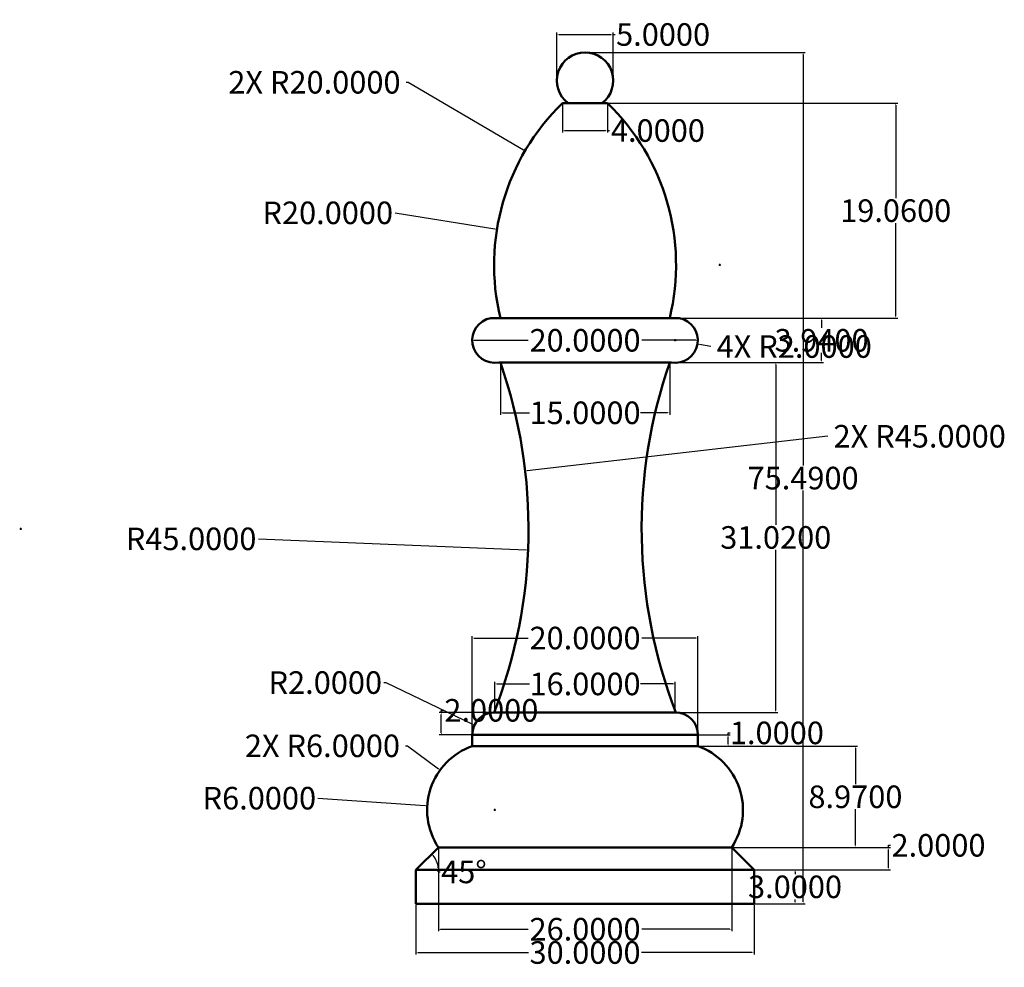
# Model space of a CAD drawing. Units: inches. Extents: x 2555.6 to 2642.8, y 681.4 to 765.4.
import ezdxf

# ---------------------------------------------------------------- set-up
doc = ezdxf.new("R2010")
doc.units = ezdxf.units.IN
doc.header["$MEASUREMENT"] = 0
doc.layers.add('M-DIMS', color=2, linetype='Continuous', lineweight=25)
doc.layers.add('M-OUTL', color=7, linetype='Continuous', lineweight=50)
doc.styles.get("Standard").update_dxf_attribs({"font": 'arial.ttf'})
doc.dimstyles.get("Standard").update_dxf_attribs({"dimtxt": 2, "dimasz": 0.18, "dimexe": 0.18, "dimexo": 0.0625, "dimgap": 0.09, "dimtad": 0, "dimtih": 1, "dimtoh": 1, "dimdec": 4, "dimzin": 0, "dimdsep": 46, "dimtxsty": 'Standard', "dimcen": 0.09, "dimadec": 0, "dimazin": 0, "dimtfac": 1, "dimtdec": 4, "dimtofl": 0, "dimtmove": 0, "dimatfit": 3, "dimfxl": 1, "dimtolj": 1, "dimtzin": 0, "dimarcsym": 0})

# ---------------------------------------------------------------- blocks, each defined once
blk = doc.blocks.new('*D1')
at = {"layer": 'Defpoints', "color": 0, "transparency": 16777216}
for p in [(2555.668, 720.265), (2600.629, 718.391)]:
    blk.add_point(p, dxfattribs=at)
at = {"layer": 'M-DIMS', "color": 0, "lineweight": -2, "transparency": 16777216}
blk.add_line((2576.739, 719.387), (2600.449, 718.399), dxfattribs=at)
at = {"layer": 'M-DIMS', "color": 0, "transparency": 16777216}
blk.add_solid([(2600.451, 718.429), (2600.448, 718.369), (2600.629, 718.391)], dxfattribs=at)
at = {"layer": 'M-DIMS', "color": 0, "transparency": 16777216, "insert": (2570.767, 719.387), "char_height": 2, "attachment_point": 5}
blk.add_mtext('\\A1;R45.0000', dxfattribs=at)
blk = doc.blocks.new('*D2')
at = {"layer": 'Defpoints', "color": 0, "transparency": 16777216}
for p in [(2597.869, 746.846), (2617.616, 743.676)]:
    blk.add_point(p, dxfattribs=at)
at = {"layer": 'M-DIMS', "color": 0, "lineweight": -2, "transparency": 16777216}
for p, q in [((2588.849, 748.294), (2597.691, 746.875)), ((2617.526, 743.676), (2617.706, 743.676)), ((2617.616, 743.586), (2617.616, 743.766))]:
    blk.add_line(p, q, dxfattribs=at)
at = {"layer": 'M-DIMS', "color": 0, "transparency": 16777216}
blk.add_solid([(2597.696, 746.904), (2597.687, 746.845), (2597.869, 746.846)], dxfattribs=at)
at = {"layer": 'M-DIMS', "color": 0, "transparency": 16777216, "insert": (2582.877, 748.294), "char_height": 2, "attachment_point": 5}
blk.add_mtext('\\A1;R20.0000', dxfattribs=at)
blk = doc.blocks.new('*D3')
at = {"layer": 'Defpoints', "color": 0, "transparency": 16777216}
for p in [(2595.878, 702.869), (2597.68, 702.001)]:
    blk.add_point(p, dxfattribs=at)
at = {"layer": 'M-DIMS', "color": 0, "lineweight": -2, "transparency": 16777216}
for p, q in [((2587.855, 706.643), (2588.035, 706.643)), ((2588.035, 706.643), (2595.716, 702.947)), ((2597.59, 702.001), (2597.77, 702.001)), ((2597.68, 701.911), (2597.68, 702.091))]:
    blk.add_line(p, q, dxfattribs=at)
at = {"layer": 'M-DIMS', "color": 0, "transparency": 16777216}
blk.add_solid([(2595.729, 702.974), (2595.703, 702.92), (2595.878, 702.869)], dxfattribs=at)
at = {"layer": 'M-DIMS', "color": 0, "transparency": 16777216, "insert": (2582.66, 706.643), "char_height": 2, "attachment_point": 5}
blk.add_mtext('\\A1;R2.0000', dxfattribs=at)
blk = doc.blocks.new('*D4')
at = {"layer": 'Defpoints', "color": 0, "transparency": 16777216}
for p in [(2591.695, 695.745), (2597.682, 695.345)]:
    blk.add_point(p, dxfattribs=at)
at = {"layer": 'M-DIMS', "color": 0, "lineweight": -2, "transparency": 16777216}
for p, q in [((2582.01, 696.392), (2591.516, 695.757)), ((2597.682, 695.255), (2597.682, 695.435)), ((2597.592, 695.345), (2597.772, 695.345))]:
    blk.add_line(p, q, dxfattribs=at)
at = {"layer": 'M-DIMS', "color": 0, "transparency": 16777216}
blk.add_solid([(2591.518, 695.787), (2591.514, 695.727), (2591.695, 695.745)], dxfattribs=at)
at = {"layer": 'M-DIMS', "color": 0, "transparency": 16777216, "insert": (2576.815, 696.392), "char_height": 2, "attachment_point": 5}
blk.add_mtext('\\A1;R6.0000', dxfattribs=at)
blk = doc.blocks.new('*D5')
at = {"layer": 'Defpoints', "color": 0, "transparency": 16777216}
for p in [(2592.68, 692.031), (2618.68, 692.031), (2618.68, 684.769)]:
    blk.add_point(p, dxfattribs=at)
at = {"layer": 'M-DIMS', "color": 0, "lineweight": -2, "transparency": 16777216}
for p, q in [((2592.68, 691.969), (2592.68, 684.589)), ((2618.68, 691.969), (2618.68, 684.589)), ((2592.86, 684.769), (2600.648, 684.769)), ((2618.5, 684.769), (2610.712, 684.769))]:
    blk.add_line(p, q, dxfattribs=at)
at = {"layer": 'M-DIMS', "color": 0, "transparency": 16777216}
for points in [[(2592.86, 684.799), (2592.86, 684.739), (2592.68, 684.769)], [(2618.5, 684.799), (2618.5, 684.739), (2618.68, 684.769)]]:
    blk.add_solid(points, dxfattribs=at)
at = {"layer": 'M-DIMS', "color": 0, "transparency": 16777216, "insert": (2605.68, 684.769), "char_height": 2, "attachment_point": 5}
blk.add_mtext('\\A1;26.0000', dxfattribs=at)
blk = doc.blocks.new('*D6')
at = {"layer": 'Defpoints', "color": 0, "transparency": 16777216}
for p in [(2605.68, 735.021), (2622.58, 735.021), (2605.68, 704.001)]:
    blk.add_point(p, dxfattribs=at)
at = {"layer": 'M-DIMS', "color": 0, "lineweight": -2, "transparency": 16777216}
for p, q in [((2605.743, 735.021), (2622.76, 735.021)), ((2622.58, 734.841), (2622.58, 720.623)), ((2622.58, 704.181), (2622.58, 718.399)), ((2605.743, 704.001), (2622.76, 704.001))]:
    blk.add_line(p, q, dxfattribs=at)
at = {"layer": 'M-DIMS', "color": 0, "transparency": 16777216}
for points in [[(2622.55, 734.841), (2622.61, 734.841), (2622.58, 735.021)], [(2622.55, 704.181), (2622.61, 704.181), (2622.58, 704.001)]]:
    blk.add_solid(points, dxfattribs=at)
at = {"layer": 'M-DIMS', "color": 0, "transparency": 16777216, "insert": (2622.58, 719.511), "char_height": 2, "attachment_point": 5}
blk.add_mtext('\\A1;31.0200', dxfattribs=at)
blk = doc.blocks.new('*D7')
at = {"layer": 'Defpoints', "color": 0, "transparency": 16777216}
for p in [(2605.68, 701.001), (2629.641, 701.001), (2605.68, 692.031)]:
    blk.add_point(p, dxfattribs=at)
at = {"layer": 'M-DIMS', "color": 0, "lineweight": -2, "transparency": 16777216}
for p, q in [((2605.743, 701.001), (2629.821, 701.001)), ((2629.641, 700.821), (2629.641, 697.627)), ((2629.641, 692.211), (2629.641, 695.405)), ((2605.743, 692.031), (2629.821, 692.031))]:
    blk.add_line(p, q, dxfattribs=at)
at = {"layer": 'M-DIMS', "color": 0, "transparency": 16777216}
for points in [[(2629.611, 700.821), (2629.671, 700.821), (2629.641, 701.001)], [(2629.611, 692.211), (2629.671, 692.211), (2629.641, 692.031)]]:
    blk.add_solid(points, dxfattribs=at)
at = {"layer": 'M-DIMS', "color": 0, "transparency": 16777216, "insert": (2629.641, 696.516), "char_height": 2, "attachment_point": 5}
blk.add_mtext('\\A1;8.9700', dxfattribs=at)
blk = doc.blocks.new('*D8')
at = {"layer": 'Defpoints', "color": 0, "transparency": 16777216}
for p in [(2615.767, 692.031), (2632.569, 692.031), (2615.767, 690.031)]:
    blk.add_point(p, dxfattribs=at)
at = {"layer": 'M-DIMS', "color": 0, "lineweight": -2, "transparency": 16777216}
for p, q in [((2615.829, 692.031), (2632.749, 692.031)), ((2632.569, 692.031), (2632.569, 692.211)), ((2632.569, 692.211), (2632.749, 692.211)), ((2632.569, 690.211), (2632.569, 691.851)), ((2615.829, 690.031), (2632.749, 690.031))]:
    blk.add_line(p, q, dxfattribs=at)
at = {"layer": 'M-DIMS', "color": 0, "transparency": 16777216}
for points in [[(2632.539, 691.851), (2632.599, 691.851), (2632.569, 692.031)], [(2632.539, 690.211), (2632.599, 690.211), (2632.569, 690.031)]]:
    blk.add_solid(points, dxfattribs=at)
at = {"layer": 'M-DIMS', "color": 0, "transparency": 16777216, "insert": (2637.004, 692.211), "char_height": 2, "attachment_point": 5}
blk.add_mtext('\\A1;2.0000', dxfattribs=at)
blk = doc.blocks.new('*D9')
at = {"layer": 'Defpoints', "color": 0, "transparency": 16777216}
for p in [(2620.68, 690.031), (2624.289, 690.031), (2620.68, 687.031)]:
    blk.add_point(p, dxfattribs=at)
at = {"layer": 'M-DIMS', "color": 0, "lineweight": -2, "transparency": 16777216}
for p, q in [((2620.743, 690.031), (2624.469, 690.031)), ((2624.289, 689.851), (2624.289, 689.643)), ((2620.743, 687.031), (2624.469, 687.031)), ((2624.289, 687.211), (2624.289, 687.419))]:
    blk.add_line(p, q, dxfattribs=at)
at = {"layer": 'M-DIMS', "color": 0, "transparency": 16777216}
for points in [[(2624.259, 689.851), (2624.319, 689.851), (2624.289, 690.031)], [(2624.259, 687.211), (2624.319, 687.211), (2624.289, 687.031)]]:
    blk.add_solid(points, dxfattribs=at)
at = {"layer": 'M-DIMS', "color": 0, "transparency": 16777216, "insert": (2624.289, 688.531), "char_height": 2, "attachment_point": 5}
blk.add_mtext('\\A1;3.0000', dxfattribs=at)
blk = doc.blocks.new('*D10')
at = {"layer": 'Defpoints', "color": 0, "transparency": 16777216}
for p in [(2605.68, 738.961), (2626.643, 738.961), (2605.68, 735.021)]:
    blk.add_point(p, dxfattribs=at)
at = {"layer": 'M-DIMS', "color": 0, "lineweight": -2, "transparency": 16777216}
for p, q in [((2605.743, 738.961), (2626.823, 738.961)), ((2626.643, 738.781), (2626.643, 738.103)), ((2626.643, 735.201), (2626.643, 735.879)), ((2605.743, 735.021), (2626.823, 735.021))]:
    blk.add_line(p, q, dxfattribs=at)
at = {"layer": 'M-DIMS', "color": 0, "transparency": 16777216}
for points in [[(2626.613, 738.781), (2626.673, 738.781), (2626.643, 738.961)], [(2626.613, 735.201), (2626.673, 735.201), (2626.643, 735.021)]]:
    blk.add_solid(points, dxfattribs=at)
at = {"layer": 'M-DIMS', "color": 0, "transparency": 16777216, "insert": (2626.643, 736.991), "char_height": 2, "attachment_point": 5}
blk.add_mtext('\\A1;3.9400', dxfattribs=at)
blk = doc.blocks.new('*D11')
at = {"layer": 'Defpoints', "color": 0, "transparency": 16777216}
for p in [(2605.68, 758.021), (2633.212, 758.021), (2605.68, 738.961)]:
    blk.add_point(p, dxfattribs=at)
at = {"layer": 'M-DIMS', "color": 0, "lineweight": -2, "transparency": 16777216}
for p, q in [((2605.743, 758.021), (2633.392, 758.021)), ((2633.212, 757.841), (2633.212, 749.602)), ((2633.212, 739.141), (2633.212, 747.38)), ((2605.743, 738.961), (2633.392, 738.961))]:
    blk.add_line(p, q, dxfattribs=at)
at = {"layer": 'M-DIMS', "color": 0, "transparency": 16777216}
for points in [[(2633.182, 757.841), (2633.242, 757.841), (2633.212, 758.021)], [(2633.182, 739.141), (2633.242, 739.141), (2633.212, 738.961)]]:
    blk.add_solid(points, dxfattribs=at)
at = {"layer": 'M-DIMS', "color": 0, "transparency": 16777216, "insert": (2633.212, 748.491), "char_height": 2, "attachment_point": 5}
blk.add_mtext('\\A1;19.0600', dxfattribs=at)
blk = doc.blocks.new('*D12')
at = {"layer": 'Defpoints', "color": 0, "transparency": 16777216}
for p in [(2608.18, 764.109), (2603.18, 760.021), (2608.18, 760.021)]:
    blk.add_point(p, dxfattribs=at)
at = {"layer": 'M-DIMS', "color": 0, "lineweight": -2, "transparency": 16777216}
for p, q in [((2603.18, 760.084), (2603.18, 764.289)), ((2603.36, 764.109), (2608, 764.109)), ((2608.18, 760.084), (2608.18, 764.289)), ((2608.18, 764.109), (2608.36, 764.109))]:
    blk.add_line(p, q, dxfattribs=at)
at = {"layer": 'M-DIMS', "color": 0, "transparency": 16777216}
for points in [[(2603.36, 764.139), (2603.36, 764.079), (2603.18, 764.109)], [(2608, 764.139), (2608, 764.079), (2608.18, 764.109)]]:
    blk.add_solid(points, dxfattribs=at)
at = {"layer": 'M-DIMS', "color": 0, "transparency": 16777216, "insert": (2612.598, 764.109), "char_height": 2, "attachment_point": 5}
blk.add_mtext('\\A1;5.0000', dxfattribs=at)
blk = doc.blocks.new('*D13')
at = {"layer": 'Defpoints', "color": 0, "transparency": 16777216}
for p in [(2598.18, 735.021), (2613.18, 735.021), (2613.18, 730.565)]:
    blk.add_point(p, dxfattribs=at)
at = {"layer": 'M-DIMS', "color": 0, "lineweight": -2, "transparency": 16777216}
for p, q in [((2598.18, 734.959), (2598.18, 730.385)), ((2613.18, 734.959), (2613.18, 730.385)), ((2598.36, 730.565), (2600.759, 730.565)), ((2613, 730.565), (2610.601, 730.565))]:
    blk.add_line(p, q, dxfattribs=at)
at = {"layer": 'M-DIMS', "color": 0, "transparency": 16777216}
for points in [[(2598.36, 730.595), (2598.36, 730.535), (2598.18, 730.565)], [(2613, 730.595), (2613, 730.535), (2613.18, 730.565)]]:
    blk.add_solid(points, dxfattribs=at)
at = {"layer": 'M-DIMS', "color": 0, "transparency": 16777216, "insert": (2605.68, 730.565), "char_height": 2, "attachment_point": 5}
blk.add_mtext('\\A1;15.0000', dxfattribs=at)
blk = doc.blocks.new('*D14')
at = {"layer": 'Defpoints', "color": 0, "transparency": 16777216}
for p in [(2595.68, 736.991), (2615.68, 736.991), (2615.68, 736.991)]:
    blk.add_point(p, dxfattribs=at)
at = {"layer": 'M-DIMS', "color": 0, "lineweight": -2, "transparency": 16777216}
for p, q in [((2595.68, 737.054), (2595.68, 737.171)), ((2595.86, 736.991), (2600.648, 736.991)), ((2615.5, 736.991), (2610.712, 736.991)), ((2615.68, 737.054), (2615.68, 737.171))]:
    blk.add_line(p, q, dxfattribs=at)
at = {"layer": 'M-DIMS', "color": 0, "transparency": 16777216}
for points in [[(2595.86, 737.021), (2595.86, 736.961), (2595.68, 736.991)], [(2615.5, 737.021), (2615.5, 736.961), (2615.68, 736.991)]]:
    blk.add_solid(points, dxfattribs=at)
at = {"layer": 'M-DIMS', "color": 0, "transparency": 16777216, "insert": (2605.68, 736.991), "char_height": 2, "attachment_point": 5}
blk.add_mtext('\\A1;20.0000', dxfattribs=at)
blk = doc.blocks.new('*D15')
at = {"layer": 'Defpoints', "color": 0, "transparency": 16777216}
for p in [(2613.68, 706.522), (2597.68, 704.001), (2613.68, 704.001)]:
    blk.add_point(p, dxfattribs=at)
at = {"layer": 'M-DIMS', "color": 0, "lineweight": -2, "transparency": 16777216}
for p, q in [((2597.68, 704.064), (2597.68, 706.702)), ((2597.86, 706.522), (2600.759, 706.522)), ((2613.5, 706.522), (2610.601, 706.522)), ((2613.68, 704.064), (2613.68, 706.702))]:
    blk.add_line(p, q, dxfattribs=at)
at = {"layer": 'M-DIMS', "color": 0, "transparency": 16777216}
for points in [[(2597.86, 706.552), (2597.86, 706.492), (2597.68, 706.522)], [(2613.5, 706.552), (2613.5, 706.492), (2613.68, 706.522)]]:
    blk.add_solid(points, dxfattribs=at)
at = {"layer": 'M-DIMS', "color": 0, "transparency": 16777216, "insert": (2605.68, 706.522), "char_height": 2, "attachment_point": 5}
blk.add_mtext('\\A1;16.0000', dxfattribs=at)
blk = doc.blocks.new('*D16')
at = {"layer": 'Defpoints', "color": 0, "transparency": 16777216}
for p in [(2615.68, 710.592), (2595.68, 702.001), (2615.68, 702.001)]:
    blk.add_point(p, dxfattribs=at)
at = {"layer": 'M-DIMS', "color": 0, "lineweight": -2, "transparency": 16777216}
for p, q in [((2595.68, 702.064), (2595.68, 710.772)), ((2595.86, 710.592), (2600.648, 710.592)), ((2615.5, 710.592), (2610.712, 710.592)), ((2615.68, 702.064), (2615.68, 710.772))]:
    blk.add_line(p, q, dxfattribs=at)
at = {"layer": 'M-DIMS', "color": 0, "transparency": 16777216}
for points in [[(2595.86, 710.622), (2595.86, 710.562), (2595.68, 710.592)], [(2615.5, 710.622), (2615.5, 710.562), (2615.68, 710.592)]]:
    blk.add_solid(points, dxfattribs=at)
at = {"layer": 'M-DIMS', "color": 0, "transparency": 16777216, "insert": (2605.68, 710.592), "char_height": 2, "attachment_point": 5}
blk.add_mtext('\\A1;20.0000', dxfattribs=at)
blk = doc.blocks.new('*D17')
at = {"layer": 'Defpoints', "color": 0, "transparency": 16777216}
for p in [(2592.68, 692.031), (2592.412, 691.031), (2590.68, 690.031), (2590.68, 690.031), (2620.68, 690.031)]:
    blk.add_point(p, dxfattribs=at)
at = {"layer": 'M-DIMS', "color": 0, "lineweight": -2, "transparency": 16777216}
blk.add_line((2592.672, 689.852), (2592.852, 689.852), dxfattribs=at)
for start, end in [(5.15836, 39.84164), (354.84164, 360)]:
    blk.add_arc((2590.68, 690.031), 2, start, end, dxfattribs=at)
at = {"layer": 'M-DIMS', "color": 0, "transparency": 16777216}
for points in [[(2592.194, 691.292), (2592.238, 691.333), (2592.094, 691.446)], [(2592.702, 690.212), (2592.642, 690.21), (2592.68, 690.031)]]:
    blk.add_solid(points, dxfattribs=at)
at = {"layer": 'M-DIMS', "color": 0, "transparency": 16777216, "insert": (2594.944, 689.852), "char_height": 2, "attachment_point": 5}
blk.add_mtext('\\A1;45°', dxfattribs=at)
blk = doc.blocks.new('*D18')
at = {"layer": 'Defpoints', "color": 0, "transparency": 16777216}
for p in [(2615.68, 702.001), (2618.355, 702.001), (2615.68, 701.001)]:
    blk.add_point(p, dxfattribs=at)
at = {"layer": 'M-DIMS', "color": 0, "lineweight": -2, "transparency": 16777216}
for p, q in [((2615.743, 702.001), (2618.535, 702.001)), ((2618.355, 702.001), (2618.355, 702.181)), ((2618.355, 702.181), (2618.535, 702.181)), ((2618.355, 701.181), (2618.355, 701.821)), ((2615.743, 701.001), (2618.535, 701.001))]:
    blk.add_line(p, q, dxfattribs=at)
at = {"layer": 'M-DIMS', "color": 0, "transparency": 16777216}
for points in [[(2618.325, 701.821), (2618.385, 701.821), (2618.355, 702.001)], [(2618.325, 701.181), (2618.385, 701.181), (2618.355, 701.001)]]:
    blk.add_solid(points, dxfattribs=at)
at = {"layer": 'M-DIMS', "color": 0, "transparency": 16777216, "insert": (2622.679, 702.181), "char_height": 2, "attachment_point": 5}
blk.add_mtext('\\A1;1.0000', dxfattribs=at)
blk = doc.blocks.new('*D19')
at = {"layer": 'Defpoints', "color": 0, "transparency": 16777216}
for p in [(2592.943, 704.001), (2604.037, 704.001), (2604.037, 702.001)]:
    blk.add_point(p, dxfattribs=at)
at = {"layer": 'M-DIMS', "color": 0, "lineweight": -2, "transparency": 16777216}
for p, q in [((2592.943, 704.001), (2592.943, 704.181)), ((2592.943, 704.181), (2593.123, 704.181)), ((2603.975, 704.001), (2592.763, 704.001)), ((2592.943, 702.181), (2592.943, 703.821)), ((2603.975, 702.001), (2592.763, 702.001))]:
    blk.add_line(p, q, dxfattribs=at)
at = {"layer": 'M-DIMS', "color": 0, "transparency": 16777216}
for points in [[(2592.913, 703.821), (2592.973, 703.821), (2592.943, 704.001)], [(2592.913, 702.181), (2592.973, 702.181), (2592.943, 702.001)]]:
    blk.add_solid(points, dxfattribs=at)
at = {"layer": 'M-DIMS', "color": 0, "transparency": 16777216, "insert": (2597.378, 704.181), "char_height": 2, "attachment_point": 5}
blk.add_mtext('\\A1;2.0000', dxfattribs=at)
blk = doc.blocks.new('*D20')
at = {"layer": 'Defpoints', "color": 0, "transparency": 16777216}
for p in [(2603.68, 758.021), (2607.68, 758.021), (2607.68, 755.591)]:
    blk.add_point(p, dxfattribs=at)
at = {"layer": 'M-DIMS', "color": 0, "lineweight": -2, "transparency": 16777216}
for p, q in [((2603.68, 757.959), (2603.68, 755.411)), ((2607.68, 757.959), (2607.68, 755.411)), ((2603.86, 755.591), (2607.5, 755.591)), ((2607.68, 755.591), (2607.86, 755.591))]:
    blk.add_line(p, q, dxfattribs=at)
at = {"layer": 'M-DIMS', "color": 0, "transparency": 16777216}
for points in [[(2603.86, 755.621), (2603.86, 755.561), (2603.68, 755.591)], [(2607.5, 755.621), (2607.5, 755.561), (2607.68, 755.591)]]:
    blk.add_solid(points, dxfattribs=at)
at = {"layer": 'M-DIMS', "color": 0, "transparency": 16777216, "insert": (2612.138, 755.591), "char_height": 2, "attachment_point": 5}
blk.add_mtext('\\A1;4.0000', dxfattribs=at)
blk = doc.blocks.new('*D21')
at = {"layer": 'Defpoints', "color": 0, "transparency": 16777216}
for p in [(2605.68, 762.521), (2620.68, 687.031), (2625.005, 687.031)]:
    blk.add_point(p, dxfattribs=at)
at = {"layer": 'M-DIMS', "color": 0, "lineweight": -2, "transparency": 16777216}
for p, q in [((2605.743, 762.521), (2625.185, 762.521)), ((2625.005, 762.341), (2625.005, 725.887)), ((2625.005, 687.211), (2625.005, 723.665)), ((2620.743, 687.031), (2625.185, 687.031))]:
    blk.add_line(p, q, dxfattribs=at)
at = {"layer": 'M-DIMS', "color": 0, "transparency": 16777216}
for points in [[(2624.975, 762.341), (2625.035, 762.341), (2625.005, 762.521)], [(2624.975, 687.211), (2625.035, 687.211), (2625.005, 687.031)]]:
    blk.add_solid(points, dxfattribs=at)
at = {"layer": 'M-DIMS', "color": 0, "transparency": 16777216, "insert": (2625.005, 724.776), "char_height": 2, "attachment_point": 5}
blk.add_mtext('\\A1;75.4900', dxfattribs=at)
blk = doc.blocks.new('*D22')
at = {"layer": 'Defpoints', "color": 0, "transparency": 16777216}
for p in [(2590.68, 687.031), (2620.68, 687.031), (2620.68, 682.706)]:
    blk.add_point(p, dxfattribs=at)
at = {"layer": 'M-DIMS', "color": 0, "lineweight": -2, "transparency": 16777216}
for p, q in [((2590.68, 686.969), (2590.68, 682.526)), ((2620.68, 686.969), (2620.68, 682.526)), ((2590.86, 682.706), (2600.666, 682.706)), ((2620.5, 682.706), (2610.694, 682.706))]:
    blk.add_line(p, q, dxfattribs=at)
at = {"layer": 'M-DIMS', "color": 0, "transparency": 16777216}
for points in [[(2590.86, 682.736), (2590.86, 682.676), (2590.68, 682.706)], [(2620.5, 682.736), (2620.5, 682.676), (2620.68, 682.706)]]:
    blk.add_solid(points, dxfattribs=at)
at = {"layer": 'M-DIMS', "color": 0, "transparency": 16777216, "insert": (2605.68, 682.706), "char_height": 2, "attachment_point": 5}
blk.add_mtext('\\A1;30.0000', dxfattribs=at)
blk = doc.blocks.new('*D23')
at = {"layer": 'Defpoints', "color": 0, "transparency": 16777216}
for p in [(2600.366, 753.797), (2617.616, 743.676)]:
    blk.add_point(p, dxfattribs=at)
at = {"layer": 'M-DIMS', "color": 0, "lineweight": -2, "transparency": 16777216}
for p, q in [((2589.836, 759.87), (2590.016, 759.87)), ((2590.016, 759.87), (2600.211, 753.888)), ((2617.526, 743.676), (2617.706, 743.676)), ((2617.616, 743.586), (2617.616, 743.766))]:
    blk.add_line(p, q, dxfattribs=at)
at = {"layer": 'M-DIMS', "color": 0, "transparency": 16777216}
blk.add_solid([(2600.226, 753.914), (2600.196, 753.862), (2600.366, 753.797)], dxfattribs=at)
at = {"layer": 'M-DIMS', "color": 0, "transparency": 16777216, "insert": (2581.698, 759.87), "char_height": 2, "attachment_point": 5}
blk.add_mtext('\\A1;2X R20.0000', dxfattribs=at)
blk = doc.blocks.new('*D24')
at = {"layer": 'Defpoints', "color": 0, "transparency": 16777216}
for p in [(2600.374, 725.403), (2555.668, 720.265)]:
    blk.add_point(p, dxfattribs=at)
at = {"layer": 'M-DIMS', "color": 0, "lineweight": -2, "transparency": 16777216}
for p, q in [((2627.197, 728.485), (2600.553, 725.423)), ((2555.578, 720.265), (2555.758, 720.265)), ((2555.668, 720.175), (2555.668, 720.355))]:
    blk.add_line(p, q, dxfattribs=at)
at = {"layer": 'M-DIMS', "color": 0, "transparency": 16777216}
blk.add_solid([(2600.549, 725.453), (2600.556, 725.393), (2600.374, 725.403)], dxfattribs=at)
at = {"layer": 'M-DIMS', "color": 0, "transparency": 16777216, "insert": (2635.335, 728.485), "char_height": 2, "attachment_point": 5}
blk.add_mtext('\\A1;2X R45.0000', dxfattribs=at)
blk = doc.blocks.new('*D25')
at = {"layer": 'Defpoints', "color": 0, "transparency": 16777216}
for p in [(2592.849, 698.901), (2597.682, 695.345)]:
    blk.add_point(p, dxfattribs=at)
at = {"layer": 'M-DIMS', "color": 0, "lineweight": -2, "transparency": 16777216}
for p, q in [((2589.769, 701.034), (2589.949, 701.034)), ((2589.949, 701.034), (2592.704, 699.007)), ((2597.682, 695.255), (2597.682, 695.435)), ((2597.592, 695.345), (2597.772, 695.345))]:
    blk.add_line(p, q, dxfattribs=at)
at = {"layer": 'M-DIMS', "color": 0, "transparency": 16777216}
blk.add_solid([(2592.722, 699.032), (2592.686, 698.983), (2592.849, 698.901)], dxfattribs=at)
at = {"layer": 'M-DIMS', "color": 0, "transparency": 16777216, "insert": (2582.408, 701.034), "char_height": 2, "attachment_point": 5}
blk.add_mtext('\\A1;2X R6.0000', dxfattribs=at)
blk = doc.blocks.new('*D26')
at = {"layer": 'Defpoints', "color": 0, "transparency": 16777216}
for p in [(2613.68, 736.991), (2615.65, 736.646)]:
    blk.add_point(p, dxfattribs=at)
at = {"layer": 'M-DIMS', "color": 0, "lineweight": -2, "transparency": 16777216}
for p, q in [((2613.59, 736.991), (2613.77, 736.991)), ((2613.68, 736.901), (2613.68, 737.081)), ((2616.832, 736.439), (2615.827, 736.615))]:
    blk.add_line(p, q, dxfattribs=at)
at = {"layer": 'M-DIMS', "color": 0, "transparency": 16777216}
blk.add_solid([(2615.832, 736.644), (2615.822, 736.585), (2615.65, 736.646)], dxfattribs=at)
at = {"layer": 'M-DIMS', "color": 0, "transparency": 16777216, "insert": (2624.216, 736.439), "char_height": 2, "attachment_point": 5}
blk.add_mtext('\\A1;4X R2.0000', dxfattribs=at)

msp = doc.modelspace()

# ---------------------------------------------------------------- linework, layer by layer
at = {"layer": 'M-OUTL'}
for p, q in [((2603.68005, 758.02133), (2607.68005, 758.02133)), ((2603.68005, 758.02133), (2607.68005, 758.02133)), ((2598.18005, 738.96133), (2597.33495, 738.96133)), ((2598.18005, 738.96133), (2613.18005, 738.96133)), ((2613.18005, 738.96133), (2614.02516, 738.96133)), ((2598.02516, 735.02133), (2613.33495, 735.02133)), ((2597.68005, 704.00133), (2613.68005, 704.00133)), ((2595.68005, 702.00133), (2615.68005, 702.00133)), ((2595.68005, 702.00133), (2595.68005, 701.00133)), ((2615.68005, 702.00133), (2615.68005, 701.00133)), ((2595.68005, 701.00133), (2615.68005, 701.00133)), ((2592.68005, 692.03133), (2590.68005, 690.03133)), ((2592.68005, 692.03133), (2618.68005, 692.03133)), ((2618.68005, 692.03133), (2620.68005, 690.03133)), ((2590.68005, 690.03133), (2620.68005, 690.03133)), ((2590.68005, 690.03133), (2590.68005, 687.03133)), ((2620.68005, 690.03133), (2620.68005, 687.03133)), ((2590.68005, 687.03133), (2592.68005, 687.03133)), ((2592.68005, 687.03133), (2620.68005, 687.03133))]:
    msp.add_line(p, q, dxfattribs=at)
for centre, radius, start, end in [((2605.68005, 760.02133), 2.5, 306.8698976, 233.1301024), ((2617.61634, 743.67629), 20, 134.1719587, 193.6357352), ((2593.74377, 743.67629), 20, 346.3642648, 45.8280413), ((2597.68005, 736.99133), 2, 99.9363671, 279.9363671), ((2613.68005, 736.99133), 2, 260.0636329, 80.0636329), ((2555.66815, 720.26538), 45, 338.8113585, 19.1419619), ((2655.69196, 720.26538), 45, 160.8580381, 201.1886415), ((2597.68005, 702.00133), 2, 90, 180), ((2613.68005, 702.00133), 2, 0, 90), ((2597.68192, 695.34513), 6, 109.4901441, 213.5250219), ((2613.67819, 695.34513), 6, 326.4749781, 70.5098559)]:
    msp.add_arc(centre, radius, start, end, dxfattribs=at)

# ---------------------------------------------------------------- dimensions: what is measured, and where the dimension line sits
at = {"layer": 'M-DIMS'}
for base, p1, p2, override, picture, middle in [((2608.18005, 764.10928), (2603.18005, 760.02133), (2608.18005, 760.02133), {"dimclrd": 0, "dimclre": 0, "dimclrt": 0}, '*D12', (2612.59808, 764.10928)), ((2607.68005, 755.5907), (2603.68005, 758.02133), (2607.68005, 758.02133), {"dimclrd": 0, "dimclre": 0, "dimclrt": 0}, '*D20', (2612.13832, 755.5907)), ((2615.68005, 736.99133), (2595.68005, 736.99133), (2615.68005, 736.99133), {"dimclrd": 0, "dimclre": 0, "dimclrt": 0}, '*D14', (2605.68005, 736.99133)), ((2613.18005, 730.56464), (2598.18005, 735.02133), (2613.18005, 735.02133), {"dimclrd": 0, "dimclre": 0, "dimclrt": 0}, '*D13', (2605.68005, 730.56464)), ((2615.68005, 710.5918), (2595.68005, 702.00133), (2615.68005, 702.00133), {"dimclrd": 0, "dimclre": 0, "dimclrt": 0}, '*D16', (2605.68005, 710.5918)), ((2613.68005, 706.52229), (2597.68005, 704.00133), (2613.68005, 704.00133), {"dimclrd": 0, "dimclre": 0, "dimclrt": 0}, '*D15', (2605.68005, 706.52229)), ((2618.68005, 684.76855), (2592.68005, 692.03133), (2618.68005, 692.03133), {"dimclrd": 0, "dimclre": 0, "dimclrt": 0}, '*D5', (2605.68005, 684.76855)), ((2620.68005, 682.70633), (2590.68005, 687.03133), (2620.68005, 687.03133), {"dimdec": 4, "dimlfac": 1, "dimrnd": 0, "dimzin": 0, "dimdsep": 46, "dimlunit": 2}, '*D22', (2605.68005, 682.70633))]:
    dim = msp.add_linear_dim(base=base, p1=p1, p2=p2, dimstyle='Standard', override=override, dxfattribs=at)
    dim.commit()
    dim.dimension.update_dxf_attribs({"geometry": picture, "text_midpoint": middle})
for center, mpoint, text, picture, middle in [((2617.61634, 743.67629), (2600.36617, 753.79715), '2X <>', '*D23', (2581.69833, 759.86967)), ((2613.68005, 736.99133), (2615.65002, 736.646), '4X <>', '*D26', (2616.83199, 736.4388)), ((2555.66815, 720.26538), (2600.37394, 725.40275), '2X <>', '*D24', (2627.19741, 728.48517)), ((2597.68192, 695.34513), (2592.84896, 698.90076), '2X <>', '*D25', (2582.40838, 701.03414))]:
    dim = msp.add_radius_dim(center=center, mpoint=mpoint, text=text, dimstyle='Standard', override={"dimdec": 4, "dimlfac": 1, "dimrnd": 0, "dimzin": 0, "dimdsep": 46, "dimlunit": 2}, dxfattribs=at)
    dim.commit()
    dim.dimension.update_dxf_attribs({"geometry": picture, "text_midpoint": middle, "dimtype": 164})
for base, p1, p2, override, picture, middle in [((2625.00505, 687.03133), (2605.68005, 762.52133), (2620.68005, 687.03133), {"dimdec": 4, "dimlfac": 1, "dimrnd": 0, "dimzin": 0, "dimdsep": 46, "dimlunit": 2}, '*D21', (2625.00505, 724.77633)), ((2633.2118, 758.02133), (2605.68005, 738.96133), (2605.68005, 758.02133), {"dimclrd": 0, "dimclre": 0, "dimclrt": 0}, '*D11', (2633.2118, 748.49133)), ((2626.64315, 738.96133), (2605.68005, 735.02133), (2605.68005, 738.96133), {"dimclrd": 0, "dimclre": 0, "dimclrt": 0}, '*D10', (2626.64315, 736.99133)), ((2622.57996, 735.02133), (2605.68005, 704.00133), (2605.68005, 735.02133), {"dimclrd": 0, "dimclre": 0, "dimclrt": 0}, '*D6', (2622.57996, 719.51133)), ((2592.94333, 704.00133), (2604.03747, 702.00133), (2604.03747, 704.00133), {"dimclrd": 0, "dimclre": 0, "dimclrt": 0}, '*D19', (2597.37841, 704.18133)), ((2618.35519, 702.00133), (2615.68005, 701.00133), (2615.68005, 702.00133), {"dimclrd": 0, "dimclre": 0, "dimclrt": 0}, '*D18', (2622.67908, 702.18133)), ((2629.64065, 701.00133), (2605.68005, 692.03133), (2605.68005, 701.00133), {"dimclrd": 0, "dimclre": 0, "dimclrt": 0}, '*D7', (2629.64065, 696.51633)), ((2632.56866, 692.03133), (2615.76665, 690.03133), (2615.76665, 692.03133), {"dimclrd": 0, "dimclre": 0, "dimclrt": 0}, '*D8', (2637.00373, 692.21133)), ((2624.28891, 690.03133), (2620.68005, 687.03133), (2620.68005, 690.03133), {"dimclrd": 0, "dimclre": 0, "dimclrt": 0}, '*D9', (2624.28891, 688.53133))]:
    dim = msp.add_linear_dim(base=base, p1=p1, p2=p2, angle=90, dimstyle='Standard', override=override, dxfattribs=at)
    dim.commit()
    dim.dimension.update_dxf_attribs({"geometry": picture, "text_midpoint": middle})
for center, mpoint, picture, middle in [((2617.61634, 743.67629), (2597.86914, 746.84619), '*D2', (2588.84921, 748.2941)), ((2555.66815, 720.26538), (2600.62911, 718.39128), '*D1', (2576.73895, 719.38709)), ((2597.68005, 702.00133), (2595.87786, 702.86856), '*D3', (2582.65996, 706.64262)), ((2597.68192, 695.34513), (2591.69528, 695.74521), '*D4', (2582.01003, 696.39245))]:
    dim = msp.add_radius_dim(center=center, mpoint=mpoint, dimstyle='Standard', override={"dimclrd": 0, "dimclre": 0, "dimclrt": 0}, dxfattribs=at)
    dim.commit()
    dim.dimension.update_dxf_attribs({"geometry": picture, "text_midpoint": middle, "dimtype": 164})
dim = msp.add_angular_dim_2l(base=(2592.41211, 691.03133), line1=((2590.68005, 690.03133), (2620.68005, 690.03133)), line2=((2592.68005, 692.03133), (2590.68005, 690.03133)), dimstyle='Standard', override={"dimclrd": 0, "dimclre": 0, "dimclrt": 0}, dxfattribs=at)
dim.commit()
dim.dimension.update_dxf_attribs({"geometry": '*D17', "text_midpoint": (2594.944, 689.85151)})

doc.saveas('drawing.dxf')
